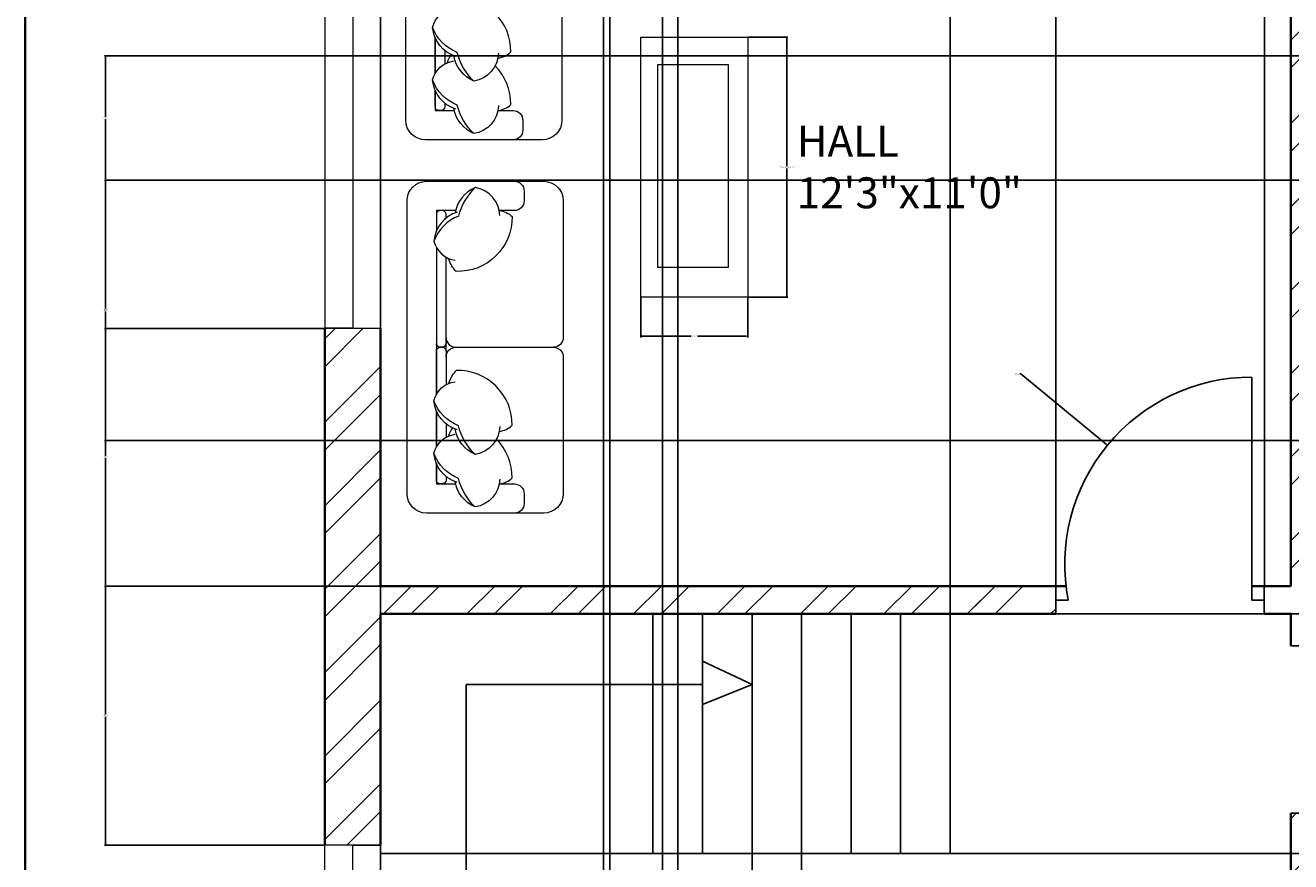
# Model space of a CAD drawing. Units: inches. Extents: x 2529 to 3014, y 1203 to 2262.
# Tile 4 of 13: x 2529 to 2733, y 1873 to 2008. Entities that reach past the tile are written whole.
import ezdxf

# ---------------------------------------------------------------- set-up
doc = ezdxf.new("R2010")
doc.units = ezdxf.units.IN
for name, color, linetype, lineweight in [('A-ANNO-DIMS', 2, 'Continuous', 18), ('A-ANNO-TTLB', 7, 'Continuous', 35), ('A-AREA-IDEN', 7, 'Continuous', 18), ('A-DOOR', 21, 'Continuous', 25), ('A-FLOR-STRS', 61, 'Continuous', 25), ('A-FURN', 8, 'Continuous', 18), ('A-GLAZ', 191, 'Continuous', 18), ('A-WALL', 7, 'Continuous', 35), ('A-WALL-PATT', 143, 'Continuous', 13)]:
    doc.layers.add(name, color=color, linetype=linetype, lineweight=lineweight)
doc.styles.get("Standard").update_dxf_attribs({"font": 'arial.ttf'})
doc.dimstyles.get("Standard").update_dxf_attribs({"dimtxt": 0.18, "dimasz": 0.18, "dimexe": 0.18, "dimexo": 0.0625, "dimgap": 0.09, "dimtad": 0, "dimtih": 1, "dimtoh": 1, "dimdec": 4, "dimzin": 0, "dimdsep": 46, "dimtxsty": 'Standard', "dimcen": 0.09, "dimadec": 0, "dimazin": 0, "dimtfac": 1, "dimtdec": 4, "dimtofl": 0, "dimtmove": 0, "dimatfit": 3, "dimfxl": 1, "dimtolj": 1, "dimtzin": 0, "dimarcsym": 0})

# ---------------------------------------------------------------- blocks, each defined once
blk = doc.blocks.new('WIN-60x9')
for p, q in [((0, 60), (9, 60)), ((0, 60), (0, 0)), ((9, 60), (4.5, 60)), ((4.5, 60), (4.5, 0)), ((9, 60), (9, 0)), ((4.5, 0), (0, 0)), ((0, 0), (9, 0))]:
    blk.add_line(p, q)
blk = doc.blocks.new('TABLE-COFFEE')
for points in [[(0, 41.99), (17.26, 41.99), (17.26, 0), (0, 0)], [(2.75, 37.58), (14.12, 37.58), (14.12, 4.82), (2.75, 4.82)]]:
    blk.add_lwpolyline(points, close=True)
blk = doc.blocks.new('*D14')
at = {"layer": 'A-ANNO-DIMS', "color": 0, "lineweight": -2, "transparency": 16777216}
for p, q in [((2645.42, 2006.13), (2651.84, 2006.13)), ((2651.66, 2005.95), (2651.66, 1985.32)), ((2651.66, 1964.32), (2651.66, 1984.95)), ((2645.42, 1964.14), (2651.84, 1964.14))]:
    blk.add_line(p, q, dxfattribs=at)
at = {"layer": 'A-ANNO-DIMS', "color": 0, "transparency": 16777216}
for points in [[(2651.63, 2005.95), (2651.69, 2005.95), (2651.66, 2006.13)], [(2651.63, 1964.32), (2651.69, 1964.32), (2651.66, 1964.14)]]:
    blk.add_solid(points, dxfattribs=at)
at = {"layer": 'Defpoints', "color": 0, "transparency": 16777216}
for p in [(2645.36, 2006.13), (2651.66, 2006.13), (2645.36, 1964.14)]:
    blk.add_point(p, dxfattribs=at)
at = {"layer": 'A-ANNO-DIMS', "color": 0, "transparency": 16777216, "insert": (2651.66, 1985.13), "char_height": 0.18, "attachment_point": 5}
blk.add_mtext('\\A1;COFFEE TABLE 42 TYP.', dxfattribs=at)
blk = doc.blocks.new('*D15')
at = {"layer": 'A-ANNO-DIMS', "color": 0, "lineweight": -2, "transparency": 16777216}
for p, q in [((2628.1, 1964.08), (2628.1, 1957.66)), ((2645.36, 1964.08), (2645.36, 1957.66)), ((2628.28, 1957.84), (2636.21, 1957.84)), ((2645.18, 1957.84), (2637.25, 1957.84))]:
    blk.add_line(p, q, dxfattribs=at)
at = {"layer": 'A-ANNO-DIMS', "color": 0, "transparency": 16777216}
for points in [[(2628.28, 1957.87), (2628.28, 1957.81), (2628.1, 1957.84)], [(2645.18, 1957.87), (2645.18, 1957.81), (2645.36, 1957.84)]]:
    blk.add_solid(points, dxfattribs=at)
at = {"layer": 'Defpoints', "color": 0, "transparency": 16777216}
for p in [(2628.1, 1964.14), (2645.36, 1964.14), (2645.36, 1957.84)]:
    blk.add_point(p, dxfattribs=at)
at = {"layer": 'A-ANNO-DIMS', "color": 0, "transparency": 16777216, "insert": (2636.73, 1957.84), "char_height": 0.18, "attachment_point": 5}
blk.add_mtext('\\A1;17 TYP.', dxfattribs=at)
blk = doc.blocks.new('*D25')
at = {"layer": 'A-ANNO-DIMS', "color": 0, "lineweight": -2, "transparency": 16777216}
for p, q in [((2585.99, 1917.5), (2541.45, 1917.5)), ((2541.63, 1917.32), (2541.63, 1896.77)), ((2541.63, 1875.85), (2541.63, 1896.41)), ((2576.99, 1875.67), (2541.45, 1875.67))]:
    blk.add_line(p, q, dxfattribs=at)
at = {"layer": 'A-ANNO-DIMS', "color": 0, "transparency": 16777216}
for points in [[(2541.6, 1917.32), (2541.66, 1917.32), (2541.63, 1917.5)], [(2541.6, 1875.85), (2541.66, 1875.85), (2541.63, 1875.67)]]:
    blk.add_solid(points, dxfattribs=at)
at = {"layer": 'Defpoints', "color": 0, "transparency": 16777216}
for p in [(2541.63, 1917.5), (2586.06, 1917.5), (2577.06, 1875.67)]:
    blk.add_point(p, dxfattribs=at)
at = {"layer": 'A-ANNO-DIMS', "color": 0, "transparency": 16777216, "insert": (2541.63, 1896.59), "char_height": 0.18, "attachment_point": 5}
blk.add_mtext('\\A1;41.83', dxfattribs=at)
blk = doc.blocks.new('*D26')
at = {"layer": 'A-ANNO-DIMS', "color": 0, "lineweight": -2, "transparency": 16777216}
for p, q in [((2576.99, 1959.12), (2541.45, 1959.12)), ((2541.63, 1958.94), (2541.63, 1938.49)), ((2541.63, 1917.68), (2541.63, 1938.13)), ((2585.99, 1917.5), (2541.45, 1917.5))]:
    blk.add_line(p, q, dxfattribs=at)
at = {"layer": 'A-ANNO-DIMS', "color": 0, "transparency": 16777216}
for points in [[(2541.6, 1958.94), (2541.66, 1958.94), (2541.63, 1959.12)], [(2541.6, 1917.68), (2541.66, 1917.68), (2541.63, 1917.5)]]:
    blk.add_solid(points, dxfattribs=at)
at = {"layer": 'Defpoints', "color": 0, "transparency": 16777216}
for p in [(2541.63, 1959.12), (2577.06, 1959.12), (2586.06, 1917.5)]:
    blk.add_point(p, dxfattribs=at)
at = {"layer": 'A-ANNO-DIMS', "color": 0, "transparency": 16777216, "insert": (2541.63, 1938.31), "char_height": 0.18, "attachment_point": 5}
blk.add_mtext('\\A1;41.62', dxfattribs=at)
blk = doc.blocks.new('*D32')
at = {"layer": 'A-ANNO-DIMS', "color": 0, "lineweight": -2, "transparency": 16777216}
for p, q in [((2586.06, 1826.63), (2586.06, 2243.11)), ((2586.24, 2242.93), (2603.84, 2242.93)), ((2621.88, 2242.93), (2604.27, 2242.93)), ((2622.06, 1826.63), (2622.06, 2243.11))]:
    blk.add_line(p, q, dxfattribs=at)
at = {"layer": 'A-ANNO-DIMS', "color": 0, "transparency": 16777216}
for points in [[(2586.24, 2242.96), (2586.24, 2242.9), (2586.06, 2242.93)], [(2621.88, 2242.96), (2621.88, 2242.9), (2622.06, 2242.93)]]:
    blk.add_solid(points, dxfattribs=at)
at = {"layer": 'Defpoints', "color": 0, "transparency": 16777216}
for p in [(2622.06, 2242.93), (2586.06, 1826.57), (2622.06, 1826.57)]:
    blk.add_point(p, dxfattribs=at)
at = {"layer": 'A-ANNO-DIMS', "color": 0, "transparency": 16777216, "insert": (2604.06, 2242.93), "char_height": 0.18, "attachment_point": 5}
blk.add_mtext('\\A1;36', dxfattribs=at)
blk = doc.blocks.new('*D52')
at = {"layer": 'A-ANNO-DIMS', "color": 0, "lineweight": -2, "transparency": 16777216}
for p, q in [((2695.12, 1917.57), (2695.12, 2243.11)), ((2695.3, 2242.93), (2711.5, 2242.93)), ((2728.62, 2242.93), (2712.42, 2242.93)), ((2728.8, 1917.57), (2728.8, 2243.11))]:
    blk.add_line(p, q, dxfattribs=at)
at = {"layer": 'A-ANNO-DIMS', "color": 0, "transparency": 16777216}
for points in [[(2695.3, 2242.96), (2695.3, 2242.9), (2695.12, 2242.93)], [(2728.62, 2242.96), (2728.62, 2242.9), (2728.8, 2242.93)]]:
    blk.add_solid(points, dxfattribs=at)
at = {"layer": 'Defpoints', "color": 0, "transparency": 16777216}
for p in [(2728.8, 2242.93), (2695.12, 1917.5), (2728.8, 1917.5)]:
    blk.add_point(p, dxfattribs=at)
at = {"layer": 'A-ANNO-DIMS', "color": 0, "transparency": 16777216, "insert": (2711.96, 2242.93), "char_height": 0.18, "attachment_point": 5}
blk.add_mtext('\\A1;33.673', dxfattribs=at)
blk = doc.blocks.new('*D60')
at = {"layer": 'A-ANNO-DIMS', "color": 0, "lineweight": -2, "transparency": 16777216}
for p, q in [((2918.49, 2003.13), (2541.45, 2003.13)), ((2541.63, 2002.95), (2541.63, 1993.28)), ((2541.63, 1983.24), (2541.63, 1992.91)), ((2918.49, 1983.06), (2541.45, 1983.06))]:
    blk.add_line(p, q, dxfattribs=at)
at = {"layer": 'A-ANNO-DIMS', "color": 0, "transparency": 16777216}
for points in [[(2541.6, 2002.95), (2541.66, 2002.95), (2541.63, 2003.13)], [(2541.6, 1983.24), (2541.66, 1983.24), (2541.63, 1983.06)]]:
    blk.add_solid(points, dxfattribs=at)
at = {"layer": 'Defpoints', "color": 0, "transparency": 16777216}
for p in [(2918.56, 2003.13), (2541.63, 1983.06), (2918.56, 1983.06)]:
    blk.add_point(p, dxfattribs=at)
at = {"layer": 'A-ANNO-DIMS', "color": 0, "transparency": 16777216, "insert": (2541.63, 1993.1), "char_height": 0.18, "attachment_point": 5}
blk.add_mtext('\\A1;20.077', dxfattribs=at)
blk = doc.blocks.new('*D61')
at = {"layer": 'A-ANNO-DIMS', "color": 0, "lineweight": -2, "transparency": 16777216}
for p, q in [((2918.49, 1983.06), (2541.45, 1983.06)), ((2541.63, 1982.88), (2541.63, 1962.21)), ((2541.63, 1941.18), (2541.63, 1961.85)), ((2918.49, 1941), (2541.45, 1941))]:
    blk.add_line(p, q, dxfattribs=at)
at = {"layer": 'A-ANNO-DIMS', "color": 0, "transparency": 16777216}
for points in [[(2541.6, 1982.88), (2541.66, 1982.88), (2541.63, 1983.06)], [(2541.6, 1941.18), (2541.66, 1941.18), (2541.63, 1941)]]:
    blk.add_solid(points, dxfattribs=at)
at = {"layer": 'Defpoints', "color": 0, "transparency": 16777216}
for p in [(2918.56, 1983.06), (2541.63, 1941), (2918.56, 1941)]:
    blk.add_point(p, dxfattribs=at)
at = {"layer": 'A-ANNO-DIMS', "color": 0, "transparency": 16777216, "insert": (2541.63, 1962.03), "char_height": 0.18, "attachment_point": 5}
blk.add_mtext('\\A1;42.05', dxfattribs=at)
blk = doc.blocks.new('*D65')
at = {"layer": 'A-ANNO-DIMS', "color": 0, "lineweight": -2, "transparency": 16777216}
for p, q in [((2646.06, 1874.24), (2646.06, 1483.77)), ((2654.06, 1874.24), (2654.06, 1483.77)), ((2646.24, 1483.95), (2649.91, 1483.95)), ((2653.88, 1483.95), (2650.2, 1483.95))]:
    blk.add_line(p, q, dxfattribs=at)
at = {"layer": 'A-ANNO-DIMS', "color": 0, "transparency": 16777216}
for points in [[(2646.24, 1483.98), (2646.24, 1483.92), (2646.06, 1483.95)], [(2653.88, 1483.98), (2653.88, 1483.92), (2654.06, 1483.95)]]:
    blk.add_solid(points, dxfattribs=at)
at = {"layer": 'Defpoints', "color": 0, "transparency": 16777216}
for p in [(2646.06, 1874.3), (2654.06, 1874.3), (2654.06, 1483.95)]:
    blk.add_point(p, dxfattribs=at)
at = {"layer": 'A-ANNO-DIMS', "color": 0, "transparency": 16777216, "insert": (2650.06, 1483.95), "char_height": 0.18, "attachment_point": 5}
blk.add_mtext('\\A1;8', dxfattribs=at)
blk = doc.blocks.new('*D66')
at = {"layer": 'A-ANNO-DIMS', "color": 0, "lineweight": -2, "transparency": 16777216}
for p, q in [((2622.06, 1874.36), (2622.06, 2243.11)), ((2622.24, 2242.93), (2649.84, 2242.93)), ((2677.88, 2242.93), (2650.27, 2242.93)), ((2678.06, 1874.36), (2678.06, 2243.11))]:
    blk.add_line(p, q, dxfattribs=at)
at = {"layer": 'A-ANNO-DIMS', "color": 0, "transparency": 16777216}
for points in [[(2622.24, 2242.96), (2622.24, 2242.9), (2622.06, 2242.93)], [(2677.88, 2242.96), (2677.88, 2242.9), (2678.06, 2242.93)]]:
    blk.add_solid(points, dxfattribs=at)
at = {"layer": 'Defpoints', "color": 0, "transparency": 16777216}
for p in [(2678.06, 2242.93), (2622.06, 1874.3), (2678.06, 1874.3)]:
    blk.add_point(p, dxfattribs=at)
at = {"layer": 'A-ANNO-DIMS', "color": 0, "transparency": 16777216, "insert": (2650.06, 2242.93), "char_height": 0.18, "attachment_point": 5}
blk.add_mtext('\\A1;56', dxfattribs=at)
blk = doc.blocks.new('*D67')
at = {"layer": 'A-ANNO-DIMS', "color": 0, "lineweight": -2, "transparency": 16777216}
for p, q in [((2678.12, 1913), (3007.66, 1913)), ((3007.48, 1912.82), (3007.48, 1893.83)), ((3007.48, 1874.48), (3007.48, 1893.47)), ((2678.12, 1874.3), (3007.66, 1874.3))]:
    blk.add_line(p, q, dxfattribs=at)
at = {"layer": 'A-ANNO-DIMS', "color": 0, "transparency": 16777216}
for points in [[(3007.45, 1912.82), (3007.51, 1912.82), (3007.48, 1913)], [(3007.45, 1874.48), (3007.51, 1874.48), (3007.48, 1874.3)]]:
    blk.add_solid(points, dxfattribs=at)
at = {"layer": 'Defpoints', "color": 0, "transparency": 16777216}
for p in [(2678.06, 1913), (3007.48, 1913), (2678.06, 1874.3)]:
    blk.add_point(p, dxfattribs=at)
at = {"layer": 'A-ANNO-DIMS', "color": 0, "transparency": 16777216, "insert": (3007.48, 1893.65), "char_height": 0.18, "attachment_point": 5}
blk.add_mtext('\\A1;38.7', dxfattribs=at)
blk = doc.blocks.new('*D68')
at = {"layer": 'A-ANNO-DIMS', "color": 0, "lineweight": -2, "transparency": 16777216}
for p, q in [((2622.12, 1874.3), (3007.66, 1874.3)), ((3007.48, 1874.12), (3007.48, 1850.62)), ((3007.48, 1826.75), (3007.48, 1850.25)), ((2622.12, 1826.57), (3007.66, 1826.57))]:
    blk.add_line(p, q, dxfattribs=at)
at = {"layer": 'A-ANNO-DIMS', "color": 0, "transparency": 16777216}
for points in [[(3007.45, 1874.12), (3007.51, 1874.12), (3007.48, 1874.3)], [(3007.45, 1826.75), (3007.51, 1826.75), (3007.48, 1826.57)]]:
    blk.add_solid(points, dxfattribs=at)
at = {"layer": 'Defpoints', "color": 0, "transparency": 16777216}
for p in [(2622.06, 1874.3), (3007.48, 1874.3), (2622.06, 1826.57)]:
    blk.add_point(p, dxfattribs=at)
at = {"layer": 'A-ANNO-DIMS', "color": 0, "transparency": 16777216, "insert": (3007.48, 1850.43), "char_height": 0.18, "attachment_point": 5}
blk.add_mtext('\\A1;47.735', dxfattribs=at)
blk = doc.blocks.new('*D71')
at = {"layer": 'A-ANNO-DIMS', "color": 0, "lineweight": -2, "transparency": 16777216}
for p, q in [((2623.09, 2159.68), (2623.09, 1483.77)), ((2631.58, 2159.68), (2631.58, 1483.77)), ((2623.27, 1483.95), (2626.94, 1483.95)), ((2631.4, 1483.95), (2627.73, 1483.95))]:
    blk.add_line(p, q, dxfattribs=at)
at = {"layer": 'A-ANNO-DIMS', "color": 0, "transparency": 16777216}
for points in [[(2623.27, 1483.98), (2623.27, 1483.92), (2623.09, 1483.95)], [(2631.4, 1483.98), (2631.4, 1483.92), (2631.58, 1483.95)]]:
    blk.add_solid(points, dxfattribs=at)
at = {"layer": 'Defpoints', "color": 0, "transparency": 16777216}
for p in [(2623.09, 2159.75), (2631.58, 2159.75), (2631.58, 1483.95)]:
    blk.add_point(p, dxfattribs=at)
at = {"layer": 'A-ANNO-DIMS', "color": 0, "transparency": 16777216, "insert": (2627.33, 1483.95), "char_height": 0.18, "attachment_point": 5}
blk.add_mtext('\\A1;8.484', dxfattribs=at)
blk = doc.blocks.new('*D74')
at = {"layer": 'A-ANNO-DIMS', "color": 0, "lineweight": -2, "transparency": 16777216}
for p, q in [((2622.06, 2135.91), (2622.06, 1483.77)), ((2634.06, 2135.91), (2634.06, 1483.77)), ((2622.24, 1483.95), (2627.6, 1483.95)), ((2633.88, 1483.95), (2628.51, 1483.95))]:
    blk.add_line(p, q, dxfattribs=at)
at = {"layer": 'A-ANNO-DIMS', "color": 0, "transparency": 16777216}
for points in [[(2622.24, 1483.98), (2622.24, 1483.92), (2622.06, 1483.95)], [(2633.88, 1483.98), (2633.88, 1483.92), (2634.06, 1483.95)]]:
    blk.add_solid(points, dxfattribs=at)
at = {"layer": 'Defpoints', "color": 0, "transparency": 16777216}
for p in [(2622.06, 2135.98), (2634.06, 2135.98), (2634.06, 1483.95)]:
    blk.add_point(p, dxfattribs=at)
at = {"layer": 'A-ANNO-DIMS', "color": 0, "transparency": 16777216, "insert": (2628.06, 1483.95), "char_height": 0.18, "attachment_point": 5}
blk.add_mtext('\\A1;12.002', dxfattribs=at)
blk = doc.blocks.new('*D82')
at = {"layer": 'A-ANNO-DIMS', "color": 0, "lineweight": -2, "transparency": 16777216}
for p, q in [((2689.29, 1951.79), (2689.47, 1951.79)), ((2689.47, 1951.79), (2703.33, 1940.37)), ((2726.71, 1921.02), (2726.89, 1921.02)), ((2726.8, 1920.93), (2726.8, 1921.11))]:
    blk.add_line(p, q, dxfattribs=at)
at = {"layer": 'A-ANNO-DIMS', "color": 0, "transparency": 16777216}
blk.add_solid([(2703.35, 1940.39), (2703.31, 1940.34), (2703.47, 1940.25)], dxfattribs=at)
at = {"layer": 'Defpoints', "color": 0, "transparency": 16777216}
for p in [(2703.47, 1940.25), (2726.8, 1921.02)]:
    blk.add_point(p, dxfattribs=at)
at = {"layer": 'A-ANNO-DIMS', "color": 0, "transparency": 16777216, "insert": (2688.81, 1951.79), "char_height": 0.18, "attachment_point": 5}
blk.add_mtext('\\A1;R30.23', dxfattribs=at)

msp = doc.modelspace()

# ---------------------------------------------------------------- hatches: boundary and pattern name
at = {"layer": 'A-WALL-PATT'}
h = msp.add_hatch(dxfattribs=at)
h.set_pattern_fill('ANSI32', color=256)
h.paths.add_polyline_path([(2686.5554, 2106.5032), (2622.0554, 2106.5032), (2622.0554, 2109.2964), (2617.4223, 2109.2964), (2613.0554, 2109.2964), (2613.0554, 2106.5032), (2577.0554, 2106.5032), (2577.0554, 2092.6918), (2586.0554, 2092.6918), (2586.0554, 2102.0032), (2682.0554, 2102.0032), (2682.0554, 2099.9833), (2686.5554, 2099.9833), (2686.5554, 2102.0032)])
h.paths.add_polyline_path([(2695.2249, 2054.0032), (2686.5554, 2054.0032), (2686.5554, 2080.2316), (2684.3054, 2080.2316), (2682.0554, 2080.2316), (2682.0554, 2054.0032), (2586.0554, 2054.0032), (2586.0554, 2068.6918), (2577.0554, 2068.6918), (2577.0554, 2019.1229), (2586.0554, 2019.1229), (2586.0554, 2049.5032), (2695.2249, 2049.5032)])
h.paths.add_polyline_path([(2737.5554, 2049.5032), (2866.5554, 2049.5032), (2866.5554, 2045.0233), (2871.0554, 2045.0233), (2871.0554, 2049.5032), (2871.0554, 2172.5032), (2866.5554, 2172.5032), (2829.1265, 2172.5032), (2829.1265, 2168.0032), (2866.5554, 2168.0032), (2866.5554, 2054.0032), (2737.5554, 2054.0032), (2737.5554, 2056.4892), (2735.3054, 2056.4892), (2733.0554, 2056.4892), (2733.0554, 2049.5032), (2733.0554, 1917.5032), (2733.0554, 1913.0032), (2871.0554, 1913.0032), (2871.0554, 1924.9149), (2868.8054, 1924.9149), (2866.5554, 1924.9149), (2866.5554, 1917.5032), (2737.5554, 1917.5032)], flags=17)
h.paths.add_polyline_path([(2972.0554, 2207.5032), (2613.0554, 2207.5032), (2613.0554, 2205.5032), (2613.0554, 2188.9366), (2622.0554, 2188.9366), (2622.0554, 2198.5032), (2733.0554, 2198.5032), (2733.0554, 2084.8053), (2735.3054, 2084.8053), (2737.5554, 2084.8053), (2737.5554, 2168.0032), (2769.1265, 2168.0032), (2769.1265, 2170.2532), (2769.1265, 2172.5032), (2737.5554, 2172.5032), (2737.5554, 2198.5032), (2963.0554, 2198.5032), (2963.0554, 2093.5032), (2912.0586, 2093.5032), (2912.0586, 2089.0032), (2918.5554, 2089.0032), (2918.5554, 2031.8749), (2923.0554, 2031.8749), (2923.0554, 2089.0032), (2963.0554, 2089.0032), (2963.0554, 2010.0032), (2923.0554, 2010.0032), (2923.0554, 2011.9417), (2918.5554, 2011.9417), (2918.5554, 2003.1338), (2923.0554, 2003.1338), (2923.0554, 2005.5032), (2963.0554, 2005.5032), (2963.0554, 1917.5032), (2963.0554, 1691.0776), (2972.0554, 1691.0776), (2972.0554, 1917.5032)])
h.paths.add_polyline_path([(2963.0554, 1945.5032), (2923.0554, 1945.5032), (2923.0554, 1983.0571), (2920.8054, 1983.0571), (2918.5554, 1983.0571), (2918.5554, 1941.0032), (2963.0554, 1941.0032)], flags=17)
h.paths.add_polyline_path([(2930.3679, 1788.7532), (2930.3679, 1791.0032), (2894.8637, 1791.0032), (2894.8637, 1786.5032), (2900.5554, 1786.5032), (2900.5554, 1784.6931), (2905.0554, 1784.6931), (2905.0554, 1786.5032), (2930.3679, 1786.5032)], flags=17)
h.paths.add_polyline_path([(2963.0554, 1791.0032), (2954.3679, 1791.0032), (2954.3679, 1786.5032), (2963.0554, 1786.5032)], flags=17)
h.paths.add_polyline_path([(2871.0554, 1853.0032), (2919.0554, 1853.0032), (2919.0554, 1847.0972), (2923.5554, 1847.0972), (2923.5554, 1853.0032), (2923.5554, 1857.5032), (2871.0554, 1857.5032), (2871.0554, 1871.7024), (2866.5554, 1871.7024), (2866.5554, 1791.0032), (2737.5554, 1791.0032), (2737.5554, 1806.6712), (2735.3054, 1806.6712), (2733.0554, 1806.6712), (2733.0554, 1791.0032), (2733.0554, 1786.5032), (2733.0554, 1780.6235), (2737.5554, 1780.6235), (2737.5554, 1786.5032), (2872.8745, 1786.5032), (2872.8745, 1788.7532), (2872.8745, 1791.0032), (2871.0554, 1791.0032)], flags=17)
h.paths.add_polyline_path([(2844.0554, 1734.0032), (2848.2652, 1734.0032), (2848.2652, 1738.5032), (2800.0167, 1738.5032), (2800.0167, 1734.0032), (2839.5554, 1734.0032), (2839.5554, 1582.5032), (2792.3334, 1582.5032), (2792.3334, 1573.5032), (2871.4433, 1573.5032), (2871.4433, 1578.0032), (2871.4433, 1582.5032), (2844.0554, 1582.5032)])
h.paths.add_polyline_path([(2972.0554, 1631.0776), (2963.0554, 1631.0776), (2963.0554, 1582.5032), (2931.4433, 1582.5032), (2931.4433, 1573.5032), (2972.0554, 1573.5032)])
h.paths.add_polyline_path([(2756.3334, 1582.5032), (2737.5554, 1582.5032), (2737.5554, 1734.0032), (2744.3201, 1734.0032), (2744.3201, 1738.5032), (2737.5554, 1738.5032), (2737.5554, 1746.0094), (2733.0554, 1746.0094), (2733.0554, 1738.5032), (2733.0554, 1612.5032), (2728.2475, 1612.5032), (2728.2475, 1603.5032), (2733.0554, 1603.5032), (2733.0554, 1582.5032), (2733.0554, 1573.5032), (2756.3334, 1573.5032), (2756.3334, 1578.0032)])
h.paths.add_polyline_path([(2695.7662, 1612.5032), (2658.4771, 1612.5032), (2658.4771, 1603.5032), (2695.7662, 1603.5032), (2695.7662, 1608.0032)])
h.paths.add_polyline_path([(2586.0554, 1686.9483), (2577.0554, 1686.9483), (2577.0554, 1603.5032), (2598.4771, 1603.5032), (2598.4771, 1608.0032), (2598.4771, 1612.5032), (2586.0554, 1612.5032)])
h.paths.add_polyline_path([(2683.2727, 1791.0032), (2586.0554, 1791.0032), (2586.0554, 1815.6736), (2581.5554, 1815.6736), (2577.0554, 1815.6736), (2577.0554, 1746.9483), (2586.0554, 1746.9483), (2586.0554, 1786.5032), (2683.2727, 1786.5032)])
h.paths.add_polyline_path([(2586.0554, 1959.1229), (2577.0554, 1959.1229), (2577.0554, 1875.6736), (2586.0554, 1875.6736), (2586.0554, 1913.0032), (2683.2727, 1913.0032), (2683.2727, 1917.5032), (2586.0554, 1917.5032)])
h = msp.add_hatch(dxfattribs=at)
h.set_pattern_fill('ANSI32', color=256)
h.paths.add_polyline_path([(2737.5554, 1786.5032), (2872.8745, 1786.5032), (2872.8745, 1788.7532), (2872.8745, 1791.0032), (2871.0554, 1791.0032), (2871.0554, 1853.0032), (2919.0554, 1853.0032), (2919.0554, 1847.0972), (2923.5554, 1847.0972), (2923.5554, 1853.0032), (2923.5554, 1857.5032), (2871.0554, 1857.5032), (2871.0554, 1871.7024), (2866.5554, 1871.7024), (2866.5554, 1791.0032), (2737.5554, 1791.0032), (2737.5554, 1806.6712), (2735.3054, 1806.6712), (2733.0554, 1806.6712), (2733.0554, 1791.0032), (2730.085, 1791.0032), (2730.085, 1786.5032), (2733.0554, 1786.5032), (2733.0554, 1780.6235), (2737.5554, 1780.6235)])
h.paths.add_polyline_path([(2737.5554, 1880.8133), (2735.3054, 1880.8133), (2733.0554, 1880.8133), (2733.0554, 1854.6712), (2737.5554, 1854.6712)])
h.paths.add_polyline_path([(2695.1228, 1915.2532), (2695.1228, 1917.5032), (2586.0554, 1917.5032), (2586.0554, 1959.1229), (2577.0554, 1959.1229), (2577.0554, 1875.6736), (2586.0554, 1875.6736), (2586.0554, 1913.0032), (2695.1228, 1913.0032)])

# ---------------------------------------------------------------- linework, layer by layer
at = {"layer": 'A-ANNO-TTLB'}
msp.add_lwpolyline([(2528.6765, 2261.8165), (3013.6003, 2261.8165), (3013.6003, 1455.1523), (2528.6765, 1455.1523)], close=True, dxfattribs=at)
at = {"layer": 'A-DOOR'}
for p, q in [((2726.7963, 1915.2532), (2726.7963, 1951.2532)), ((2695.1228, 1917.5032), (2695.1228, 1913.0032)), ((2728.7963, 1917.5032), (2728.7963, 1913.0032)), ((2695.1228, 1913.0032), (2695.1228, 1915.2532)), ((2695.1228, 1915.2532), (2697.1228, 1915.2532)), ((2728.7963, 1915.2532), (2726.7963, 1915.2532)), ((2728.7963, 1913.0032), (2728.7963, 1915.2532)), ((2733.0554, 1907.8704), (2737.5554, 1907.8704)), ((2733.0554, 1880.8133), (2737.5554, 1880.8133))]:
    msp.add_line(p, q, dxfattribs=at)
msp.add_arc((2726.7963, 1921.0239), 30.2294, 90, 191.004986, dxfattribs=at)
at = {"layer": 'A-FLOR-STRS'}
for p, q in [((2622.0554, 1874.3024), (2622.0554, 1913.0032)), ((2630.0554, 1874.3024), (2630.0554, 1913.0032)), ((2638.0554, 1874.3024), (2638.0554, 1913.0032)), ((2646.0554, 1874.3024), (2646.0554, 1913.0032)), ((2654.0554, 1874.3024), (2654.0554, 1913.0032)), ((2662.0554, 1874.3024), (2662.0554, 1913.0032)), ((2670.0554, 1874.3024), (2670.0554, 1913.0032)), ((2678.0554, 1874.3024), (2678.0554, 1913.0032)), ((2646.0554, 1901.5876), (2638.0554, 1905.3918)), ((2638.0554, 1905.3918), (2638.0554, 1897.2906)), ((2599.8977, 1806.4779), (2599.8977, 1901.5876)), ((2599.8977, 1901.5876), (2638.0554, 1901.5876)), ((2638.0554, 1898.3774), (2646.0554, 1901.5876)), ((2638.0554, 1897.2906), (2638.0554, 1898.3774)), ((2622.0554, 1874.3024), (2586.0554, 1874.3024)), ((2586.0554, 1874.3024), (2678.0554, 1874.3024)), ((2622.0554, 1826.5675), (2622.0554, 1874.3024))]:
    msp.add_line(p, q, dxfattribs=at)
at = {"layer": 'A-FURN', "ltscale": 0.03}
for points in [[(2615.3428, 2014.7731, -0.41421356), (2613.7668, 2013.1971, -0.41421356), (2615.3428, 2011.621), (2615.3428, 1992.7085, -0.41421356), (2612.1907, 1989.5564), (2593.2781, 1989.5564, -0.41421356), (2590.126, 1992.7085), (2590.126, 2033.6857, -0.41421356), (2593.2781, 2036.8378), (2612.1907, 2036.8378, -0.41421356), (2615.3428, 2033.6857), (2615.3428, 2014.7731, -0.41421356), (2613.7668, 2013.1971, -0.41421356), (2615.3428, 2011.621)], [(2615.5545, 1957.6406, -0.41421356), (2613.9785, 1956.0645, -0.41421356), (2615.5545, 1954.4885), (2615.5545, 1932.4238, -0.41421356), (2612.4025, 1929.2717), (2593.4899, 1929.2717, -0.41421356), (2590.3378, 1932.4238), (2590.3378, 1979.7052, -0.41421356), (2593.4899, 1982.8573), (2612.4025, 1982.8573, -0.41421356), (2615.5545, 1979.7052), (2615.5545, 1957.6406, -0.41421356), (2613.9785, 1956.0645, -0.41421356), (2615.5545, 1954.4885)]]:
    msp.add_lwpolyline(points, format="xyb", dxfattribs=at)
at = {"layer": 'A-FURN'}
for points in [[(2605.02, 2002.7712, 0.16554063), (2607.1024, 2003.7462, 0.42598917), (2598.0737, 2012.5976, 0.12152332), (2596.8293, 2010.4964, -7.11546429)], [(2598.219, 2003.0195, -0.30666349), (2594.4623, 2007.7203, -0.30632997), (2597.8932, 2010.7912, 0.87284716)], [(2601.1435, 1999.0495, -0.14772988), (2598.4349, 2003.6559, -0.21334276), (2594.4623, 2007.7203, -0.17866181)], [(2594.8542, 2000.222), (2594.8542, 2006.0902, -0.41421356)], [(2596.4302, 2003.9773), (2596.4302, 2001.809, -0.41421356)], [(2597.4454, 2003.3276, 0.07186538), (2596.8293, 2002.0063, -7.11546429)], [(2605.1161, 2003.5655, -0.35677236), (2601.1435, 1999.0495, -0.24954205), (2597.8697, 2003.1414, 9.61688035)], [(2598.219, 1994.5294, -0.30666349), (2594.4623, 1999.2302, -0.30632997), (2597.8932, 2002.301, 0.87284716)], [(2605.02, 1994.2811, 0.16554063), (2607.1024, 1995.2561, 0.20023115), (2604.5662, 2001.5124, 0.12152332)], [(2601.1435, 1990.5594, -0.14772988), (2598.4349, 1995.1657, -0.21334276), (2594.4623, 1999.2302, -0.17866181)], [(2594.8542, 1994.9149), (2594.8542, 1997.6001, -0.41421356)], [(2594.8542, 1997.6001), (2594.8542, 1994.2845), (2597.9515, 1994.2845, -0.41421356)], [(2596.4302, 1995.4872), (2596.4302, 1994.9149, -0.41421356), (2595.7998, 1994.2845), (2595.4846, 1994.2845, -0.41421356), (2594.8542, 1994.9149)], [(2605.1161, 1995.0754, -0.35677236), (2601.1435, 1990.5594, -0.24954205), (2597.8697, 1994.6513, 9.61688035)], [(2605.0207, 1994.2845), (2607.4626, 1994.2845, -0.41421356), (2609.0386, 1992.7085), (2609.0386, 1991.1324, -0.41421356), (2607.4626, 1989.5564)], [(2607.6743, 1982.8573, -0.41421356), (2609.2504, 1981.2813), (2609.2504, 1979.7052, -0.41421356), (2607.6743, 1978.1292), (2605.2324, 1978.1292)], [(2601.3552, 1981.8543, 0.14772988), (2598.6466, 1977.2479, 0.21334276), (2594.674, 1973.1835, 0.17866181)], [(2605.3278, 1977.3383, 0.35677236), (2601.3552, 1981.8543, 0.24954205), (2598.0814, 1977.7624, -9.61688035)], [(2598.4307, 1977.8843, 0.30666349), (2594.674, 1973.1835, 0.30632997), (2598.1049, 1970.1126, -0.87284716)], [(2596.642, 1976.9265), (2596.642, 1977.4988, 0.41421356), (2596.0115, 1978.1292), (2595.6963, 1978.1292, 0.41421356), (2595.0659, 1977.4988)], [(2595.0659, 1977.4988), (2595.0659, 1974.8136, 0.41421356)], [(2605.2317, 1978.1326, -0.16554063), (2607.3141, 1977.1576, -0.42598917), (2598.2855, 1968.3062, -0.12152332), (2597.041, 1970.4074, 7.11546429)], [(2595.0659, 1972.1917), (2595.0659, 1956.6949, 0.41421356), (2595.6963, 1956.0645), (2596.0115, 1956.0645, 0.41421356), (2596.642, 1956.6949), (2596.642, 1970.6047, 0.41421356)], [(2595.0659, 1948.4275), (2595.0659, 1955.4341, -0.41421356), (2595.6963, 1956.0645), (2596.0115, 1956.0645, -0.41421356), (2596.642, 1955.4341), (2596.642, 1950.0145, -0.41421356)], [(2596.642, 1957.6406, 0.41421356), (2598.218, 1956.0645)], [(2596.642, 1957.6406, 0.41421356), (2598.218, 1956.0645), (2613.9785, 1956.0645, 0.41421356)], [(2596.642, 1954.4885, -0.41421356), (2598.218, 1956.0645)], [(2596.642, 1954.4885, -0.41421356), (2598.218, 1956.0645), (2613.9785, 1956.0645, -0.41421356)], [(2605.2317, 1942.4865, 0.16554063), (2607.3141, 1943.4615, 0.42598917), (2598.2855, 1952.3129, 0.12152332), (2597.041, 1950.2118, -7.11546429)], [(2598.4307, 1942.7348, -0.30666349), (2594.674, 1947.4356, -0.30632997), (2598.1049, 1950.5065, 0.87284716)], [(2601.3552, 1938.7649, -0.14772988), (2598.6466, 1943.3712, -0.21334276), (2594.674, 1947.4356, -0.17866181)], [(2595.0659, 1939.9374), (2595.0659, 1945.8055, -0.41421356)], [(2596.642, 1943.6927), (2596.642, 1941.5244, -0.41421356)], [(2598.4307, 1934.2447, -0.30666349), (2594.674, 1938.9455, -0.30632997), (2598.1049, 1942.0164, 0.87284716)], [(2597.6572, 1943.043, 0.07186538), (2597.041, 1941.7216, -7.11546429)], [(2605.3278, 1943.2809, -0.35677236), (2601.3552, 1938.7649, -0.24954205), (2598.0814, 1942.8568, 9.61688035)], [(2605.2317, 1933.9964, 0.16554063), (2607.3141, 1934.9714, 0.20023115), (2604.778, 1941.2277, 0.12152332)], [(2601.3552, 1930.2747, -0.14772988), (2598.6466, 1934.8811, -0.21334276), (2594.674, 1938.9455, -0.17866181)], [(2595.0659, 1937.3154), (2595.0659, 1933.9998), (2598.1632, 1933.9998, -0.41421356)], [(2595.0659, 1934.6303), (2595.0659, 1937.3154, -0.41421356)], [(2596.642, 1935.2025), (2596.642, 1934.6303, -0.41421356), (2596.0115, 1933.9998), (2595.6963, 1933.9998, -0.41421356), (2595.0659, 1934.6303)], [(2605.3278, 1934.7908, -0.35677236), (2601.3552, 1930.2747, -0.24954205), (2598.0814, 1934.3667, 9.61688035)], [(2605.2324, 1933.9998), (2607.6743, 1933.9998, -0.41421356), (2609.2504, 1932.4238), (2609.2504, 1930.8477, -0.41421356), (2607.6743, 1929.2717)]]:
    msp.add_lwpolyline(points, format="xyb", dxfattribs=at)
for points in [[(2594.8542, 2006.0902), (2594.8542, 2000.222)], [(2598.1632, 1978.1292), (2595.0659, 1978.1292), (2595.0659, 1974.8136)], [(2595.0659, 1972.1917), (2595.0659, 1948.4275)], [(2595.0659, 1945.8055), (2595.0659, 1939.9374)]]:
    msp.add_lwpolyline(points, dxfattribs=at)
msp.add_lwpolyline([(2595.0659, 1956.6949), (2595.0659, 1955.4341, -0.41421356), (2595.6963, 1956.0645), (2596.0115, 1956.0645, -0.41421356), (2596.642, 1955.4341), (2596.642, 1956.6949, -0.41421356), (2596.0115, 1956.0645), (2595.6963, 1956.0645, -0.41421356)], format="xyb", close=True, dxfattribs=at)
at = {"layer": 'A-WALL'}
for p, q in [((2733.0554, 2049.5032), (2733.0554, 1917.5032)), ((2577.0554, 1959.1229), (2577.0554, 1875.6736)), ((2586.0554, 1959.1229), (2586.0554, 1917.5032)), ((2586.0554, 1917.5032), (2696.7726, 1917.5032)), ((2726.7963, 1917.5032), (2733.0554, 1917.5032)), ((2586.0554, 1913.0032), (2695.1228, 1913.0032)), ((2586.0554, 1913.0032), (2586.0554, 1875.6736)), ((2728.7963, 1913.0032), (2733.0554, 1913.0032)), ((2733.0554, 1913.0032), (2733.0554, 1907.8704)), ((2733.0554, 1880.8133), (2733.0554, 1806.6712))]:
    msp.add_line(p, q, dxfattribs=at)

# ---------------------------------------------------------------- block references
at = {"layer": 'A-FURN'}
msp.add_blockref('TABLE-COFFEE', (2628.101, 1964.139), dxfattribs=at)
at = {"layer": 'A-GLAZ'}
msp.add_blockref('WIN-60x9', (2577.055, 1959.123), dxfattribs=at)
at = {"layer": 'A-GLAZ', "rotation": 180}
msp.add_blockref('WIN-60x9', (2586.0557, 1875.6735), dxfattribs=at)

# ---------------------------------------------------------------- texts
at = {"layer": 'A-AREA-IDEN', "insert": (2653.278, 1991.8401), "char_height": 5, "attachment_point": 1}
msp.add_mtext_dynamic_manual_height_columns('HALL\\P12\'3"x11\'0"', width=156.678626, gutter_width=12.5, heights=[0], dxfattribs=at)

# ---------------------------------------------------------------- dimensions: what is measured, and where the dimension line sits
at = {"layer": 'A-ANNO-DIMS'}
for base, p1, p2, override, picture, middle in [((2622.0554, 2242.9282), (2586.0554, 1826.5675), (2622.0554, 1826.5675), {"dimdec": 0, "dimlfac": 1, "dimrnd": 0, "dimzin": 0, "dimdsep": 46, "dimlunit": 2}, '*D32', (2604.0554, 2242.9282)), ((2678.0554, 2242.9282), (2622.0554, 1874.3024), (2678.0554, 1874.3024), {"dimdec": 0, "dimlfac": 1, "dimrnd": 0, "dimzin": 0, "dimdsep": 46, "dimlunit": 2}, '*D66', (2650.0554, 2242.9282)), ((2728.79627, 2242.92823), (2695.12279, 1917.50323), (2728.79627, 1917.50323), {"dimdec": 3, "dimlfac": 1, "dimrnd": 0, "dimzin": 0, "dimdsep": 46, "dimlunit": 2}, '*D52', (2711.95953, 2242.92823)), ((2631.5753, 1483.9492), (2623.0916, 2159.7466), (2631.5753, 2159.7466), {"dimdec": 3, "dimlfac": 1, "dimrnd": 0, "dimzin": 0, "dimdsep": 46, "dimlunit": 2}, '*D71', (2627.3335, 1483.9492)), ((2634.0572, 1483.9492), (2622.0554, 2135.9767), (2634.0572, 2135.9767), {"dimdec": 3, "dimlfac": 1, "dimrnd": 0, "dimzin": 0, "dimdsep": 46, "dimlunit": 2}, '*D74', (2628.0563, 1483.9492)), ((2654.0554, 1483.9492), (2646.0554, 1874.3024), (2654.0554, 1874.3024), {"dimdec": 0, "dimlfac": 1, "dimrnd": 0, "dimzin": 0, "dimdsep": 46, "dimlunit": 2}, '*D65', (2650.0554, 1483.9492))]:
    dim = msp.add_linear_dim(base=base, p1=p1, p2=p2, dimstyle='Standard', override=override, dxfattribs=at)
    dim.commit()
    dim.dimension.update_dxf_attribs({"geometry": picture, "text_midpoint": middle})
dim = msp.add_linear_dim(base=(2651.659, 2006.1297), p1=(2645.3604, 1964.1392), p2=(2645.3604, 2006.1297), angle=90, text='COFFEE TABLE <> TYP.', dimstyle='Standard', override={"dimdec": 0, "dimlfac": 1, "dimrnd": 0, "dimzin": 0, "dimdsep": 46, "dimlunit": 2}, dxfattribs=at)
dim.commit()
dim.dimension.update_dxf_attribs({"geometry": '*D14', "text_midpoint": (2651.659, 1985.1345)})
for base, p1, p2, override, picture, middle in [((2541.6304, 1983.0571), (2918.5554, 2003.1338), (2918.5554, 1983.0571), {"dimdec": 3, "dimlfac": 1, "dimrnd": 0, "dimzin": 0, "dimdsep": 46, "dimlunit": 2}, '*D60', (2541.6304, 1993.0955)), ((2541.6304, 1941.0032), (2918.5554, 1983.0571), (2918.5554, 1941.0032), {"dimdec": 2, "dimlfac": 1, "dimrnd": 0, "dimzin": 0, "dimdsep": 46, "dimlunit": 2}, '*D61', (2541.6304, 1962.0302)), ((2541.6304, 1959.1229), (2586.0554, 1917.5032), (2577.0554, 1959.1229), {"dimdec": 2, "dimlfac": 1, "dimrnd": 0, "dimzin": 0, "dimdsep": 46, "dimlunit": 2}, '*D26', (2541.6304, 1938.3131)), ((2541.6304, 1917.5032), (2577.0554, 1875.6736), (2586.0554, 1917.5032), {"dimdec": 2, "dimlfac": 1, "dimrnd": 0, "dimzin": 0, "dimdsep": 46, "dimlunit": 2}, '*D25', (2541.6304, 1896.5884)), ((3007.4804, 1913.0032), (2678.0554, 1874.3024), (2678.0554, 1913.0032), {"dimdec": 1, "dimlfac": 1, "dimrnd": 0, "dimzin": 0, "dimdsep": 46, "dimlunit": 2}, '*D67', (3007.4804, 1893.6528)), ((3007.4804, 1874.3024), (2622.0554, 1826.5675), (2622.0554, 1874.3024), {"dimdec": 3, "dimlfac": 1, "dimrnd": 0, "dimzin": 0, "dimdsep": 46, "dimlunit": 2}, '*D68', (3007.4804, 1850.435))]:
    dim = msp.add_linear_dim(base=base, p1=p1, p2=p2, angle=90, dimstyle='Standard', override=override, dxfattribs=at)
    dim.commit()
    dim.dimension.update_dxf_attribs({"geometry": picture, "text_midpoint": middle})
dim = msp.add_linear_dim(base=(2645.3604, 1957.8407), p1=(2628.1014, 1964.1392), p2=(2645.3604, 1964.1392), text='<> TYP.', dimstyle='Standard', override={"dimdec": 0, "dimlfac": 1, "dimrnd": 0, "dimzin": 0, "dimdsep": 46, "dimlunit": 2}, dxfattribs=at)
dim.commit()
dim.dimension.update_dxf_attribs({"geometry": '*D15', "text_midpoint": (2636.7309, 1957.8407)})
dim = msp.add_radius_dim(center=(2726.7963, 1921.0239), mpoint=(2703.4698, 1940.2512), dimstyle='Standard', override={"dimdec": 2, "dimlfac": 1, "dimrnd": 0, "dimzin": 0, "dimdsep": 46, "dimlunit": 2}, dxfattribs=at)
dim.commit()
dim.dimension.update_dxf_attribs({"geometry": '*D82', "text_midpoint": (2688.814, 1951.7876), "dimtype": 164})

doc.saveas('drawing.dxf')
